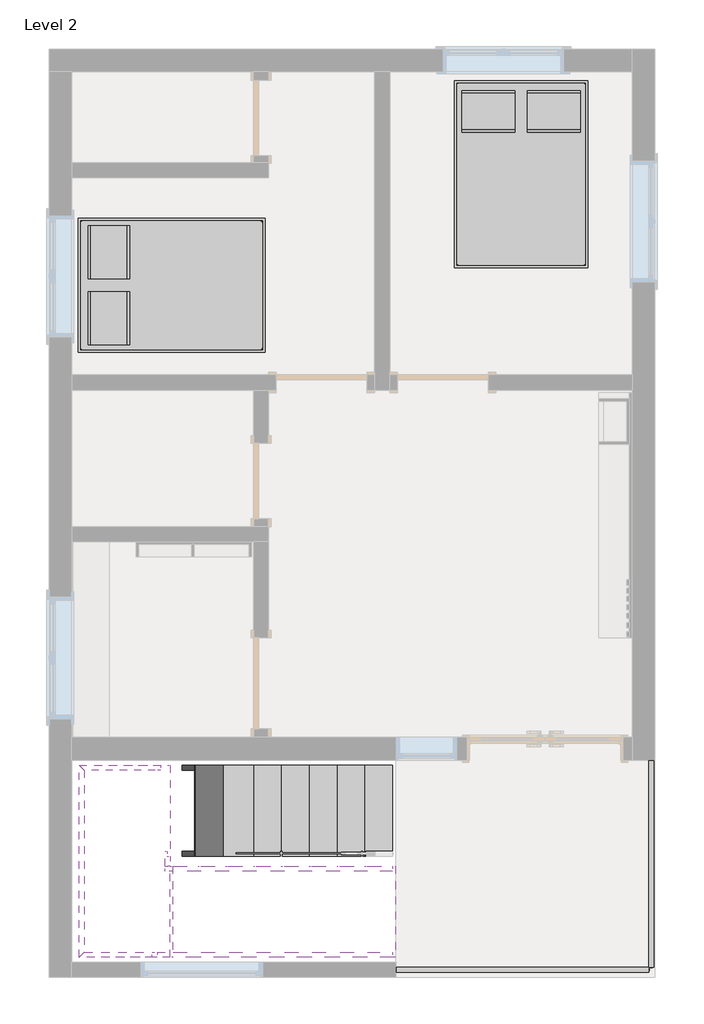
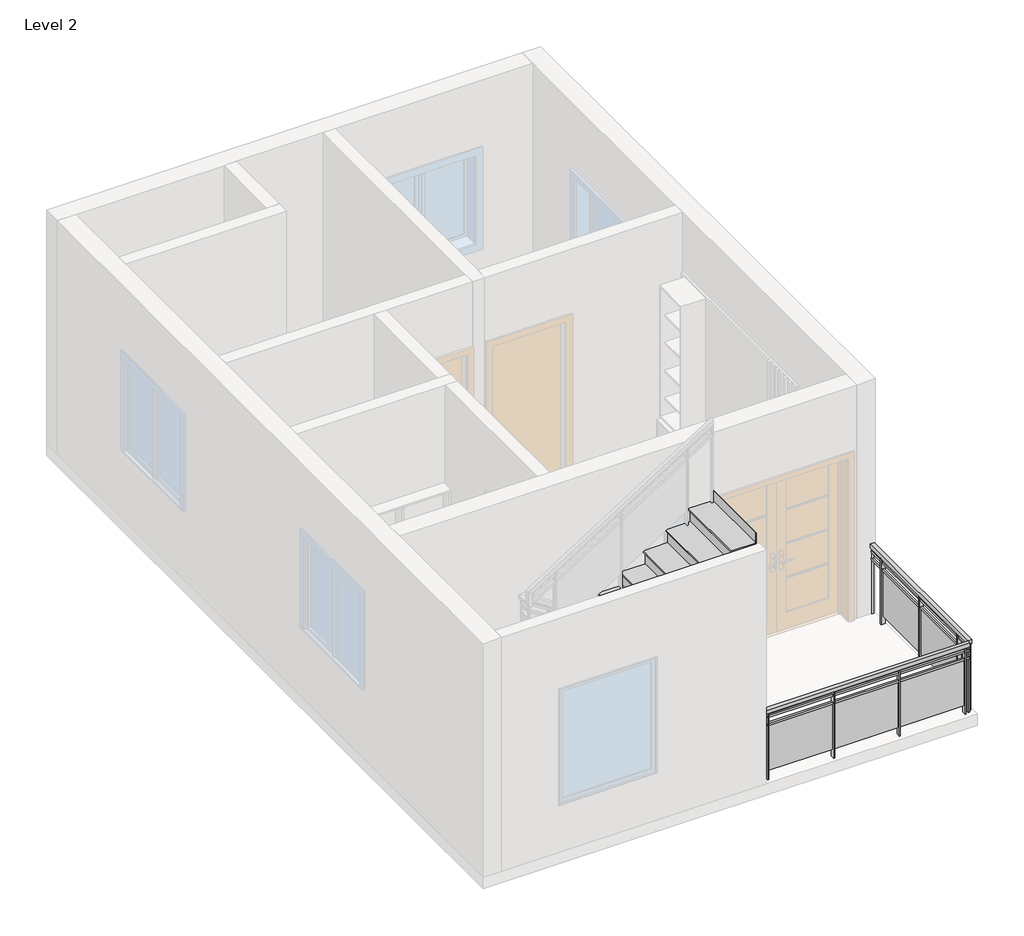
# One storey, part 2 of 2: 8 members, 2 furniture elements, 2 railings, 2 stair flights, 1 slab.
"""IFC4 building model written with IfcOpenShell, lengths in millimetres."""

from ifc_helpers import new_model, si_unit, frame, origin, place, context, project, spatial, polyline, outline, extrude, faceted_brep, transform, mapped, element, save
from components import furniture_c8abb964, non_monolithic_landing_6f2487d3, stair_flight_f94938bc, stair_flight_c7deb699

model = new_model("IFC4")

# Units and contexts
model_context = context("Model", 3, world=origin())
ifc_project = project(units=[si_unit("LENGTHUNIT", "METRE", prefix="MILLI")], contexts=[model_context])

# Site, building, storey
site = spatial("IfcSite", under=ifc_project)
building = spatial("IfcBuilding", under=site)
storey = spatial("IfcBuildingStorey", under=building, Name="Level 2", Elevation=3200.4)

# Furniture
placement = place(None, origin())
furniture_shape = furniture_c8abb964(model_context)
element("IfcFurniture", 1, ObjectType="Bed-Box : Double 53\" x 74\"", at=placement, inside=storey, context=model_context, shape_type="MappedRepresentation", body=[
    mapped(furniture_shape, transform((-5699.6768794, -383.210135, 3200.4), x_axis=(0.0, 0.9999999999999999, 0.0), y_axis=(-0.9999999999999999, 0.0, 0.0), z_axis=(0.0, 0.0, 1.0))),
])
element("IfcFurniture", 2, ObjectType="Bed-Box : Double 53\" x 74\"", at=placement, inside=storey, context=model_context, shape_type="MappedRepresentation", body=[
    mapped(furniture_shape, transform((-2286.4998302, 1307.9718322, 3200.4), x_axis=(1.0, 0.0, 0.0), y_axis=(0.0, 1.0, 0.0), z_axis=(0.0, 0.0, 1.0))),
])

# Members
element("IfcMember", 3, ObjectType="Carriage - 2\" Width", at=placement, inside=storey, context=model_context, shape_type="Brep", body=[
    faceted_brep([(-3242.7473712, -5936.857676, 6076.7282995), (-3242.7473712, -5886.057676, 6076.7282995), (-3242.7473712, -5886.057676, 6172.2), (-3242.7473712, -5936.857676, 6172.2), (-3490.3973712, -5886.057676, 5919.132845), (-3769.7973712, -5886.057676, 5741.332845), (-4049.1973712, -5886.057676, 5563.532845), (-4328.5973712, -5886.057676, 5385.732845), (-4607.9973712, -5886.057676, 5207.932845), (-4887.3973712, -5886.057676, 5030.132845), (-5166.7973712, -5886.057676, 4852.332845), (-5446.1973712, -5886.057676, 4674.532845), (-5477.9473712, -5886.057676, 4654.3282995), (-5528.7473712, -5886.057676, 4622.0010268), (-5528.7473712, -5886.057676, 4749.8), (-5477.9473712, -5886.057676, 4749.8), (-5446.1973712, -5886.057676, 4749.8), (-5446.1973712, -5886.057676, 4927.6), (-5166.7973712, -5886.057676, 4927.6), (-5166.7973712, -5886.057676, 5105.4), (-4887.3973712, -5886.057676, 5105.4), (-4887.3973712, -5886.057676, 5283.2), (-4607.9973712, -5886.057676, 5283.2), (-4607.9973712, -5886.057676, 5461.0), (-4328.5973712, -5886.057676, 5461.0), (-4328.5973712, -5886.057676, 5638.8), (-4049.1973712, -5886.057676, 5638.8), (-4049.1973712, -5886.057676, 5816.6), (-3769.7973712, -5886.057676, 5816.6), (-3769.7973712, -5886.057676, 5994.4), (-3490.3973712, -5886.057676, 5994.4), (-3490.3973712, -5886.057676, 6172.2), (-5528.7473712, -5936.857676, 4622.0010268), (-3490.3973712, -5936.857676, 6172.2), (-3490.3973712, -5936.857676, 5994.4), (-3769.7973712, -5936.857676, 5994.4), (-3769.7973712, -5936.857676, 5816.6), (-4049.1973712, -5936.857676, 5816.6), (-4049.1973712, -5936.857676, 5638.8), (-4328.5973712, -5936.857676, 5638.8), (-4328.5973712, -5936.857676, 5461.0), (-4607.9973712, -5936.857676, 5461.0), (-4607.9973712, -5936.857676, 5283.2), (-4887.3973712, -5936.857676, 5283.2), (-4887.3973712, -5936.857676, 5105.4), (-5166.7973712, -5936.857676, 5105.4), (-5166.7973712, -5936.857676, 4927.6), (-5446.1973712, -5936.857676, 4927.6), (-5446.1973712, -5936.857676, 4749.8), (-5528.7473712, -5936.857676, 4749.8)], [[[0, 1, 2, 3]], [[2, 1, 4, 5, 6, 7, 8, 9, 10, 11, 12, 13, 14, 15, 16, 17, 18, 19, 20, 21, 22, 23, 24, 25, 26, 27, 28, 29, 30, 31]], [[1, 0, 32, 13, 12, 11, 10, 9, 8, 7, 6, 5, 4]], [[32, 0, 3, 33, 34, 35, 36, 37, 38, 39, 40, 41, 42, 43, 44, 45, 46, 47, 48, 49]], [[17, 47, 46, 18]], [[47, 17, 16, 48]], [[19, 45, 44, 20]], [[18, 46, 45, 19]], [[21, 43, 42, 22]], [[20, 44, 43, 21]], [[23, 41, 40, 24]], [[22, 42, 41, 23]], [[25, 39, 38, 26]], [[24, 40, 39, 25]], [[27, 37, 36, 28]], [[26, 38, 37, 27]], [[29, 35, 34, 30]], [[28, 36, 35, 29]], [[31, 33, 3, 2]], [[30, 34, 33, 31]], [[13, 32, 49, 14]], [[48, 16, 15, 14, 49]]]),
])
element("IfcMember", 4, ObjectType="Carriage - 2\" Width", at=placement, inside=storey, context=model_context, shape_type="Brep", body=[
    faceted_brep([(-3242.7473712, -6800.457676, 6076.7282995), (-3242.7473712, -6749.657676, 6076.7282995), (-3242.7473712, -6749.657676, 6172.2), (-3242.7473712, -6800.457676, 6172.2), (-5607.3204133, -6749.657676, 4572.0), (-5659.0958955, -6749.657676, 4749.8), (-5446.1973712, -6749.657676, 4749.8), (-5446.1973712, -6749.657676, 4927.6), (-5166.7973712, -6749.657676, 4927.6), (-5166.7973712, -6749.657676, 5105.4), (-4887.3973712, -6749.657676, 5105.4), (-4887.3973712, -6749.657676, 5283.2), (-4607.9973712, -6749.657676, 5283.2), (-4607.9973712, -6749.657676, 5461.0), (-4328.5973712, -6749.657676, 5461.0), (-4328.5973712, -6749.657676, 5638.8), (-4049.1973712, -6749.657676, 5638.8), (-4049.1973712, -6749.657676, 5816.6), (-3769.7973712, -6749.657676, 5816.6), (-3769.7973712, -6749.657676, 5994.4), (-3490.3973712, -6749.657676, 5994.4), (-3490.3973712, -6749.657676, 6172.2), (-3490.3973712, -6800.457676, 5919.132845), (-3769.7973712, -6800.457676, 5741.332845), (-4049.1973712, -6800.457676, 5563.532845), (-4328.5973712, -6800.457676, 5385.732845), (-4607.9973712, -6800.457676, 5207.932845), (-4887.3973712, -6800.457676, 5030.132845), (-5166.7973712, -6800.457676, 4852.332845), (-5446.1973712, -6800.457676, 4674.532845), (-5477.9473712, -6800.457676, 4654.3282995), (-5607.3204133, -6800.457676, 4572.0), (-3490.3973712, -6800.457676, 6172.2), (-3490.3973712, -6800.457676, 5994.4), (-3769.7973712, -6800.457676, 5994.4), (-3769.7973712, -6800.457676, 5816.6), (-4049.1973712, -6800.457676, 5816.6), (-4049.1973712, -6800.457676, 5638.8), (-4328.5973712, -6800.457676, 5638.8), (-4328.5973712, -6800.457676, 5461.0), (-4607.9973712, -6800.457676, 5461.0), (-4607.9973712, -6800.457676, 5283.2), (-4887.3973712, -6800.457676, 5283.2), (-4887.3973712, -6800.457676, 5105.4), (-5166.7973712, -6800.457676, 5105.4), (-5166.7973712, -6800.457676, 4927.6), (-5446.1973712, -6800.457676, 4927.6), (-5446.1973712, -6800.457676, 4749.8), (-5477.9473712, -6800.457676, 4749.8), (-5659.0958955, -6800.457676, 4749.8)], [[[0, 1, 2, 3]], [[1, 4, 5, 6, 7, 8, 9, 10, 11, 12, 13, 14, 15, 16, 17, 18, 19, 20, 21, 2]], [[1, 0, 22, 23, 24, 25, 26, 27, 28, 29, 30, 31, 4]], [[0, 3, 32, 33, 34, 35, 36, 37, 38, 39, 40, 41, 42, 43, 44, 45, 46, 47, 48, 49, 31, 30, 29, 28, 27, 26, 25, 24, 23, 22]], [[7, 46, 45, 8]], [[46, 7, 6, 47]], [[9, 44, 43, 10]], [[8, 45, 44, 9]], [[11, 42, 41, 12]], [[10, 43, 42, 11]], [[13, 40, 39, 14]], [[12, 41, 40, 13]], [[15, 38, 37, 16]], [[14, 39, 38, 15]], [[17, 36, 35, 18]], [[16, 37, 36, 17]], [[19, 34, 33, 20]], [[18, 35, 34, 19]], [[21, 32, 3, 2]], [[20, 33, 32, 21]], [[4, 31, 49, 5]], [[47, 6, 5, 49, 48]]]),
])
element("IfcMember", 5, ObjectType="Carriage - 2\" Width", at=placement, inside=storey, context=model_context, shape_type="Brep", body=[
    faceted_brep([(-3274.4973712, -5784.457676, 3200.4), (-3472.6029006, -5784.457676, 3200.4), (-3472.6029006, -5733.657676, 3200.4), (-3274.4973712, -5733.657676, 3200.4), (-5477.9473712, -5784.457676, 4476.5282995), (-5477.9473712, -5733.657676, 4476.5282995), (-3553.8973712, -5784.457676, 3252.132845), (-3833.2973712, -5784.457676, 3429.932845), (-4112.6973712, -5784.457676, 3607.732845), (-4392.0973712, -5784.457676, 3785.532845), (-4671.4973712, -5784.457676, 3963.332845), (-4950.8973712, -5784.457676, 4141.132845), (-5230.2973712, -5784.457676, 4318.932845), (-5477.9473712, -5784.457676, 4572.0), (-3274.4973712, -5784.457676, 3327.4), (-3553.8973712, -5784.457676, 3327.4), (-3553.8973712, -5784.457676, 3505.2), (-3833.2973712, -5784.457676, 3505.2), (-3833.2973712, -5784.457676, 3683.0), (-4112.6973712, -5784.457676, 3683.0), (-4112.6973712, -5784.457676, 3860.8), (-4392.0973712, -5784.457676, 3860.8), (-4392.0973712, -5784.457676, 4038.6), (-4671.4973712, -5784.457676, 4038.6), (-4671.4973712, -5784.457676, 4216.4), (-4950.8973712, -5784.457676, 4216.4), (-4950.8973712, -5784.457676, 4394.2), (-5230.2973712, -5784.457676, 4394.2), (-5230.2973712, -5784.457676, 4572.0), (-5230.2973712, -5733.657676, 4572.0), (-5477.9473712, -5733.657676, 4572.0), (-5230.2973712, -5733.657676, 4394.2), (-4950.8973712, -5733.657676, 4394.2), (-4950.8973712, -5733.657676, 4216.4), (-4671.4973712, -5733.657676, 4216.4), (-4671.4973712, -5733.657676, 4038.6), (-4392.0973712, -5733.657676, 4038.6), (-4392.0973712, -5733.657676, 3860.8), (-4112.6973712, -5733.657676, 3860.8), (-4112.6973712, -5733.657676, 3683.0), (-3833.2973712, -5733.657676, 3683.0), (-3833.2973712, -5733.657676, 3505.2), (-3553.8973712, -5733.657676, 3505.2), (-3553.8973712, -5733.657676, 3327.4), (-3274.4973712, -5733.657676, 3327.4)], [[[0, 1, 2, 3]], [[4, 5, 2, 1, 6, 7, 8, 9, 10, 11, 12]], [[13, 4, 12, 11, 10, 9, 8, 7, 6, 1, 0, 14, 15, 16, 17, 18, 19, 20, 21, 22, 23, 24, 25, 26, 27, 28]], [[28, 29, 30, 13]], [[2, 5, 30, 29, 31, 32, 33, 34, 35, 36, 37, 38, 39, 40, 41, 42, 43, 44, 3]], [[44, 14, 0, 3]], [[14, 44, 43, 15]], [[15, 43, 42, 16]], [[16, 42, 41, 17]], [[17, 41, 40, 18]], [[18, 40, 39, 19]], [[19, 39, 38, 20]], [[20, 38, 37, 21]], [[21, 37, 36, 22]], [[22, 36, 35, 23]], [[23, 35, 34, 24]], [[24, 34, 33, 25]], [[25, 33, 32, 26]], [[26, 32, 31, 27]], [[27, 31, 29, 28]], [[5, 4, 13, 30]]]),
])
element("IfcMember", 6, ObjectType="Carriage - 2\" Width", at=placement, inside=storey, context=model_context, shape_type="Brep", body=[
    faceted_brep([(-3274.4973712, -4920.857676, 3200.4), (-3472.6029006, -4920.857676, 3200.4), (-3472.6029006, -4870.057676, 3200.4), (-3274.4973712, -4870.057676, 3200.4), (-5627.9743291, -4920.857676, 4572.0), (-5627.9743291, -4870.057676, 4572.0), (-5509.6973712, -4870.057676, 4496.732845), (-5477.9473712, -4870.057676, 4476.5282995), (-5230.2973712, -4870.057676, 4318.932845), (-4950.8973712, -4870.057676, 4141.132845), (-4671.4973712, -4870.057676, 3963.332845), (-4392.0973712, -4870.057676, 3785.532845), (-4112.6973712, -4870.057676, 3607.732845), (-3833.2973712, -4870.057676, 3429.932845), (-3553.8973712, -4870.057676, 3252.132845), (-5576.198847, -4920.857676, 4749.8), (-3274.4973712, -4920.857676, 3327.4), (-3553.8973712, -4920.857676, 3327.4), (-3553.8973712, -4920.857676, 3505.2), (-3833.2973712, -4920.857676, 3505.2), (-3833.2973712, -4920.857676, 3683.0), (-4112.6973712, -4920.857676, 3683.0), (-4112.6973712, -4920.857676, 3860.8), (-4392.0973712, -4920.857676, 3860.8), (-4392.0973712, -4920.857676, 4038.6), (-4671.4973712, -4920.857676, 4038.6), (-4671.4973712, -4920.857676, 4216.4), (-4950.8973712, -4920.857676, 4216.4), (-4950.8973712, -4920.857676, 4394.2), (-5230.2973712, -4920.857676, 4394.2), (-5230.2973712, -4920.857676, 4572.0), (-5509.6973712, -4920.857676, 4572.0), (-5509.6973712, -4920.857676, 4749.8), (-5230.2973712, -4870.057676, 4572.0), (-5477.9473712, -4870.057676, 4572.0), (-5509.6973712, -4870.057676, 4572.0), (-5576.198847, -4870.057676, 4749.8), (-5509.6973712, -4870.057676, 4749.8), (-5230.2973712, -4870.057676, 4394.2), (-4950.8973712, -4870.057676, 4394.2), (-4950.8973712, -4870.057676, 4216.4), (-4671.4973712, -4870.057676, 4216.4), (-4671.4973712, -4870.057676, 4038.6), (-4392.0973712, -4870.057676, 4038.6), (-4392.0973712, -4870.057676, 3860.8), (-4112.6973712, -4870.057676, 3860.8), (-4112.6973712, -4870.057676, 3683.0), (-3833.2973712, -4870.057676, 3683.0), (-3833.2973712, -4870.057676, 3505.2), (-3553.8973712, -4870.057676, 3505.2), (-3553.8973712, -4870.057676, 3327.4), (-3274.4973712, -4870.057676, 3327.4)], [[[0, 1, 2, 3]], [[4, 5, 6, 7, 8, 9, 10, 11, 12, 13, 14, 2, 1]], [[15, 4, 1, 0, 16, 17, 18, 19, 20, 21, 22, 23, 24, 25, 26, 27, 28, 29, 30, 31, 32]], [[30, 33, 34, 35, 31]], [[5, 36, 37, 35, 34, 33, 38, 39, 40, 41, 42, 43, 44, 45, 46, 47, 48, 49, 50, 51, 3, 2, 14, 13, 12, 11, 10, 9, 8, 7, 6]], [[51, 16, 0, 3]], [[16, 51, 50, 17]], [[17, 50, 49, 18]], [[18, 49, 48, 19]], [[19, 48, 47, 20]], [[20, 47, 46, 21]], [[21, 46, 45, 22]], [[22, 45, 44, 23]], [[23, 44, 43, 24]], [[24, 43, 42, 25]], [[25, 42, 41, 26]], [[26, 41, 40, 27]], [[27, 40, 39, 28]], [[28, 39, 38, 29]], [[29, 38, 33, 30]], [[5, 4, 15, 36]], [[31, 35, 37, 32]], [[32, 37, 36, 15]]]),
])
element("IfcMember", 7, ObjectType="Carriage - 2\" Width", at=placement, inside=storey, context=model_context, shape_type="SweptSolid", body=[
    extrude(outline(polyline([(-5528.7473712, -5886.057676), (-5528.7473712, -5733.657676), (-5509.6973712, -5733.657676), (-5509.6973712, -5784.457676), (-5477.9473712, -5784.457676), (-5477.9473712, -5886.057676), (-5528.7473712, -5886.057676)])), frame((0.0, 0.0, 4572.0), z_axis=(0.0, 0.0, 1.0), x_axis=(1.0, 0.0, 0.0)), (0.0, 0.0, 1.0), 177.8),
])
element("IfcMember", 8, ObjectType="Carriage - 2\" Width", at=placement, inside=storey, context=model_context, shape_type="Brep", body=[
    faceted_brep([(-6341.5473712, -4920.857676, 4572.0), (-5627.9743291, -4920.857676, 4572.0), (-5576.198847, -4920.857676, 4749.8), (-6341.5473712, -4920.857676, 4749.8), (-6392.3473712, -4870.057676, 4572.0), (-5627.9743291, -4870.057676, 4572.0), (-6392.3473712, -4870.057676, 4749.8), (-5576.198847, -4870.057676, 4749.8)], [[[0, 1, 2, 3]], [[1, 0, 4, 5]], [[5, 4, 6, 7]], [[3, 2, 7, 6]], [[1, 5, 7, 2]], [[4, 0, 3, 6]]]),
])
element("IfcMember", 9, ObjectType="Carriage - 2\" Width", at=placement, inside=storey, context=model_context, shape_type="SweptSolid", body=[
    extrude(outline(polyline([(-6341.5473712, -4920.857676), (-6341.5473712, -6749.657676), (-6392.3473712, -6800.457676), (-6392.3473712, -4870.057676), (-6341.5473712, -4920.857676)])), frame((0.0, 0.0, 4572.0), z_axis=(0.0, 0.0, 1.0), x_axis=(1.0, 0.0, 0.0)), (0.0, 0.0, 1.0), 177.8),
])
element("IfcMember", 10, ObjectType="Carriage - 2\" Width", at=placement, inside=storey, context=model_context, shape_type="Brep", body=[
    faceted_brep([(-5607.3204133, -6749.657676, 4572.0), (-6341.5473712, -6749.657676, 4572.0), (-6341.5473712, -6749.657676, 4749.8), (-5659.0958955, -6749.657676, 4749.8), (-5607.3204133, -6800.457676, 4572.0), (-6392.3473712, -6800.457676, 4572.0), (-5659.0958955, -6800.457676, 4749.8), (-6392.3473712, -6800.457676, 4749.8)], [[[0, 1, 2, 3]], [[1, 0, 4, 5]], [[5, 4, 6, 7]], [[3, 2, 7, 6]], [[1, 5, 7, 2]], [[4, 0, 3, 6]]]),
])

# Railings
element("IfcRailing", 11, ObjectType="Glass Panel - Bottom Fill", at=placement, inside=storey, context=model_context, shape_type="SweptSolid", body=[
    extrude(outline(polyline([(-3204.6473712, -6952.857676), (-3204.6473712, -6902.057676), (-664.6473712, -6902.057676), (-664.6473712, -6952.857676), (-3204.6473712, -6952.857676)])), frame((0.0, 0.0, 4064.0), z_axis=(0.0, 0.0, 1.0), x_axis=(1.0, 0.0, 0.0)), (0.0, 0.0, 1.0), 50.8),
    extrude(outline(polyline([(-3204.6473712, -6940.157676), (-3204.6473712, -6914.757676), (-664.6473712, -6914.757676), (-664.6473712, -6940.157676), (-3204.6473712, -6940.157676)])), frame((0.0, 0.0, 4000.5), z_axis=(0.0, 0.0, 1.0), x_axis=(1.0, 0.0, 0.0)), (0.0, 0.0, 1.0), 25.4),
    extrude(outline(polyline([(-3204.6473712, -6940.157676), (-3204.6473712, -6914.757676), (-664.6473712, -6914.757676), (-664.6473712, -6940.157676), (-3204.6473712, -6940.157676)])), frame((0.0, 0.0, 3898.9), z_axis=(0.0, 0.0, 1.0), x_axis=(1.0, 0.0, 0.0)), (0.0, 0.0, 1.0), 25.4),
    extrude(outline(polyline([(-721.7973712, -6952.857676), (-721.7973712, -6902.057676), (-709.0973712, -6902.057676), (-709.0973712, -6952.857676), (-721.7973712, -6952.857676)])), frame((0.0, 0.0, 3200.4), z_axis=(0.0, 0.0, 1.0), x_axis=(1.0, 0.0, 0.0)), (0.0, 0.0, 1.0), 863.6),
    extrude(outline(polyline([(-1528.2473712, -6920.922519), (-715.4473712, -6920.922519), (-715.4473712, -6927.272519), (-1528.2473712, -6927.272519), (-1528.2473712, -6920.922519)])), frame((0.0, 0.0, 3302.0), z_axis=(0.0, 0.0, 1.0), x_axis=(1.0, 0.0, 0.0)), (0.0, 0.0, 1.0), 596.9),
    extrude(outline(polyline([(-1534.5973712, -6952.857676), (-1534.5973712, -6902.057676), (-1521.8973712, -6902.057676), (-1521.8973712, -6952.857676), (-1534.5973712, -6952.857676)])), frame((0.0, 0.0, 3200.4), z_axis=(0.0, 0.0, 1.0), x_axis=(1.0, 0.0, 0.0)), (0.0, 0.0, 1.0), 863.6),
    extrude(outline(polyline([(-2341.0473712, -6920.922519), (-1528.2473712, -6920.922519), (-1528.2473712, -6927.272519), (-2341.0473712, -6927.272519), (-2341.0473712, -6920.922519)])), frame((0.0, 0.0, 3302.0), z_axis=(0.0, 0.0, 1.0), x_axis=(1.0, 0.0, 0.0)), (0.0, 0.0, 1.0), 596.9),
    extrude(outline(polyline([(-2347.3973712, -6952.857676), (-2347.3973712, -6902.057676), (-2334.6973712, -6902.057676), (-2334.6973712, -6952.857676), (-2347.3973712, -6952.857676)])), frame((0.0, 0.0, 3200.4), z_axis=(0.0, 0.0, 1.0), x_axis=(1.0, 0.0, 0.0)), (0.0, 0.0, 1.0), 863.6),
    extrude(outline(polyline([(-3153.8473712, -6920.922519), (-2341.0473712, -6920.922519), (-2341.0473712, -6927.272519), (-3153.8473712, -6927.272519), (-3153.8473712, -6920.922519)])), frame((0.0, 0.0, 3302.0), z_axis=(0.0, 0.0, 1.0), x_axis=(1.0, 0.0, 0.0)), (0.0, 0.0, 1.0), 596.9),
    extrude(outline(polyline([(-3160.1973712, -6952.857676), (-3160.1973712, -6902.057676), (-3147.4973712, -6902.057676), (-3147.4973712, -6952.857676), (-3160.1973712, -6952.857676)])), frame((0.0, 0.0, 3200.4), z_axis=(0.0, 0.0, 1.0), x_axis=(1.0, 0.0, 0.0)), (0.0, 0.0, 1.0), 863.6),
    extrude(outline(polyline([(-677.3473712, -6936.982676), (-677.3473712, -6917.932676), (-658.2973712, -6917.932676), (-658.2973712, -6936.982676), (-677.3473712, -6936.982676)])), frame((0.0, 0.0, 3200.4), z_axis=(0.0, 0.0, 1.0), x_axis=(1.0, 0.0, 0.0)), (0.0, 0.0, 1.0), 863.6),
    extrude(outline(polyline([(-3210.9973712, -6936.982676), (-3210.9973712, -6917.932676), (-3191.9473712, -6917.932676), (-3191.9473712, -6936.982676), (-3210.9973712, -6936.982676)])), frame((0.0, 0.0, 3200.4), z_axis=(0.0, 0.0, 1.0), x_axis=(1.0, 0.0, 0.0)), (0.0, 0.0, 1.0), 863.6),
])
element("IfcRailing", 12, ObjectType="Glass Panel - Bottom Fill", at=placement, inside=storey, context=model_context, shape_type="SweptSolid", body=[
    extrude(outline(polyline([(-664.6473712, -4819.257676), (-613.8473712, -4819.257676), (-613.8473712, -6902.057676), (-664.6473712, -6902.057676), (-664.6473712, -4819.257676)])), frame((0.0, 0.0, 4064.0), z_axis=(0.0, 0.0, 1.0), x_axis=(1.0, 0.0, 0.0)), (0.0, 0.0, 1.0), 50.8),
    extrude(outline(polyline([(-651.9473712, -4819.257676), (-626.5473712, -4819.257676), (-626.5473712, -6902.057676), (-651.9473712, -6902.057676), (-651.9473712, -4819.257676)])), frame((0.0, 0.0, 4000.5), z_axis=(0.0, 0.0, 1.0), x_axis=(1.0, 0.0, 0.0)), (0.0, 0.0, 1.0), 25.4),
    extrude(outline(polyline([(-651.9473712, -4819.257676), (-626.5473712, -4819.257676), (-626.5473712, -6902.057676), (-651.9473712, -6902.057676), (-651.9473712, -4819.257676)])), frame((0.0, 0.0, 3898.9), z_axis=(0.0, 0.0, 1.0), x_axis=(1.0, 0.0, 0.0)), (0.0, 0.0, 1.0), 25.4),
    extrude(outline(polyline([(-664.6473712, -6667.107676), (-613.8473712, -6667.107676), (-613.8473712, -6679.807676), (-664.6473712, -6679.807676), (-664.6473712, -6667.107676)])), frame((0.0, 0.0, 3200.4), z_axis=(0.0, 0.0, 1.0), x_axis=(1.0, 0.0, 0.0)), (0.0, 0.0, 1.0), 863.6),
    extrude(outline(polyline([(-632.7122142, -5860.657676), (-632.7122142, -6673.457676), (-639.0622142, -6673.457676), (-639.0622142, -5860.657676), (-632.7122142, -5860.657676)])), frame((0.0, 0.0, 3302.0), z_axis=(0.0, 0.0, 1.0), x_axis=(1.0, 0.0, 0.0)), (0.0, 0.0, 1.0), 596.9),
    extrude(outline(polyline([(-664.6473712, -5854.307676), (-613.8473712, -5854.307676), (-613.8473712, -5867.007676), (-664.6473712, -5867.007676), (-664.6473712, -5854.307676)])), frame((0.0, 0.0, 3200.4), z_axis=(0.0, 0.0, 1.0), x_axis=(1.0, 0.0, 0.0)), (0.0, 0.0, 1.0), 863.6),
    extrude(outline(polyline([(-632.7122142, -5047.857676), (-632.7122142, -5860.657676), (-639.0622142, -5860.657676), (-639.0622142, -5047.857676), (-632.7122142, -5047.857676)])), frame((0.0, 0.0, 3302.0), z_axis=(0.0, 0.0, 1.0), x_axis=(1.0, 0.0, 0.0)), (0.0, 0.0, 1.0), 596.9),
    extrude(outline(polyline([(-664.6473712, -5041.507676), (-613.8473712, -5041.507676), (-613.8473712, -5054.207676), (-664.6473712, -5054.207676), (-664.6473712, -5041.507676)])), frame((0.0, 0.0, 3200.4), z_axis=(0.0, 0.0, 1.0), x_axis=(1.0, 0.0, 0.0)), (0.0, 0.0, 1.0), 863.6),
    extrude(outline(polyline([(-648.7723712, -6889.357676), (-629.7223712, -6889.357676), (-629.7223712, -6908.407676), (-648.7723712, -6908.407676), (-648.7723712, -6889.357676)])), frame((0.0, 0.0, 3200.4), z_axis=(0.0, 0.0, 1.0), x_axis=(1.0, 0.0, 0.0)), (0.0, 0.0, 1.0), 863.6),
    extrude(outline(polyline([(-648.7723712, -4812.907676), (-629.7223712, -4812.907676), (-629.7223712, -4831.957676), (-648.7723712, -4831.957676), (-648.7723712, -4812.907676)])), frame((0.0, 0.0, 3200.4), z_axis=(0.0, 0.0, 1.0), x_axis=(1.0, 0.0, 0.0)), (0.0, 0.0, 1.0), 863.6),
])

# Slab
non_monolithic_landing_shape = non_monolithic_landing_6f2487d3(model_context)
element("IfcSlab", 13, ObjectType="Non-Monolithic Landing", at=placement, inside=storey, context=model_context, shape_type="MappedRepresentation", body=[
    mapped(non_monolithic_landing_shape, transform((0.0, 0.0, 0.0), x_axis=(1.0, 0.0, 0.0), y_axis=(0.0, 1.0, 0.0), z_axis=(0.0, 0.0, 1.0))),
])

# Stair flights
stair_flight_shape = stair_flight_f94938bc(model_context)
element("IfcStairFlight", 14, ObjectType="2\" Tread 1\" Nosing 1/4\" Riser", at=placement, inside=storey, context=model_context, shape_type="MappedRepresentation", body=[
    mapped(stair_flight_shape, transform((0.0, 0.0, 0.0), x_axis=(1.0, 0.0, 0.0), y_axis=(0.0, 1.0, 0.0), z_axis=(0.0, 0.0, 1.0))),
])
stair_flight_2_shape = stair_flight_c7deb699(model_context)
element("IfcStairFlight", 15, ObjectType="2\" Tread 1\" Nosing 1/4\" Riser", at=placement, inside=storey, context=model_context, shape_type="MappedRepresentation", body=[
    mapped(stair_flight_2_shape, transform((0.0, 0.0, 0.0), x_axis=(1.0, 0.0, 0.0), y_axis=(0.0, 1.0, 0.0), z_axis=(0.0, 0.0, 1.0))),
])

save(model, "model.ifc")

# Revit data of these elements
# Type "Bed-Box : Double 53\" x 74\""
#   Assembly Code = "E2020200"
#   Length = 6' - 2"
#   Width = 4' - 5"
#   Frame Material = Birch
#   Mattress Material = Linen, White
#   Default Elevation = 0
# Type "Glass Panel - Bottom Fill"
#   Assembly Code = "C2010400"
#   built-in parameter 1008612 = 0.0416667 (stored number, unit not read)
#   built-in parameter 1008611 = 0.0416667 (stored number, unit not read)
#   built-in parameter 1008609 = 0.333333 (stored number, unit not read)
#   built-in parameter 1008604 = 0.166667 (stored number, unit not read)
#   built-in parameter 1008603 = 0.166667 (stored number, unit not read)
#   Railing Height = 3' - 0"
#   built-in parameter 1008630 = 2
#   built-in parameter 1008610 = 2
#   built-in parameter 1008618 = Baluster - Square : 3/4"
# Elements 1, 2 (IfcFurniture, "Bed-Box : Double 53\" x 74\"")
#   Phase Created = New Construction
#   Materials on its faces: "Birch", "Linen, White"
# Elements 3, 4, 5, 6, 7, 8, 9, 10 (IfcMember, "Carriage - 2\" Width")
#   Phase Created = New Construction
# Elements 11, 12 (IfcRailing, "Glass Panel - Bottom Fill")
#   Phase Created = New Construction
#   Materials on its faces: "Glass"
# Element 13 (IfcSlab, "Non-Monolithic Landing")
#   Phase Created = New Construction
# Elements 14, 15 (IfcStairFlight, "2\" Tread 1\" Nosing 1/4\" Riser")
#   Phase Created = New Construction
# Materials
#   "Birch": class "Wood", colour RGB 224 178 126, transparency 0, Description = "Betula Alleghaniensis", Cost = 0
#   "Linen, White": class "Textile", colour RGB 247 247 239, transparency 0, Description = "Linen, white", Cost = 0
#   "Glass": class "Glass", colour RGB 0 128 192, transparency 0.75, Description = "Soda Lime Glass", Cost = 0
